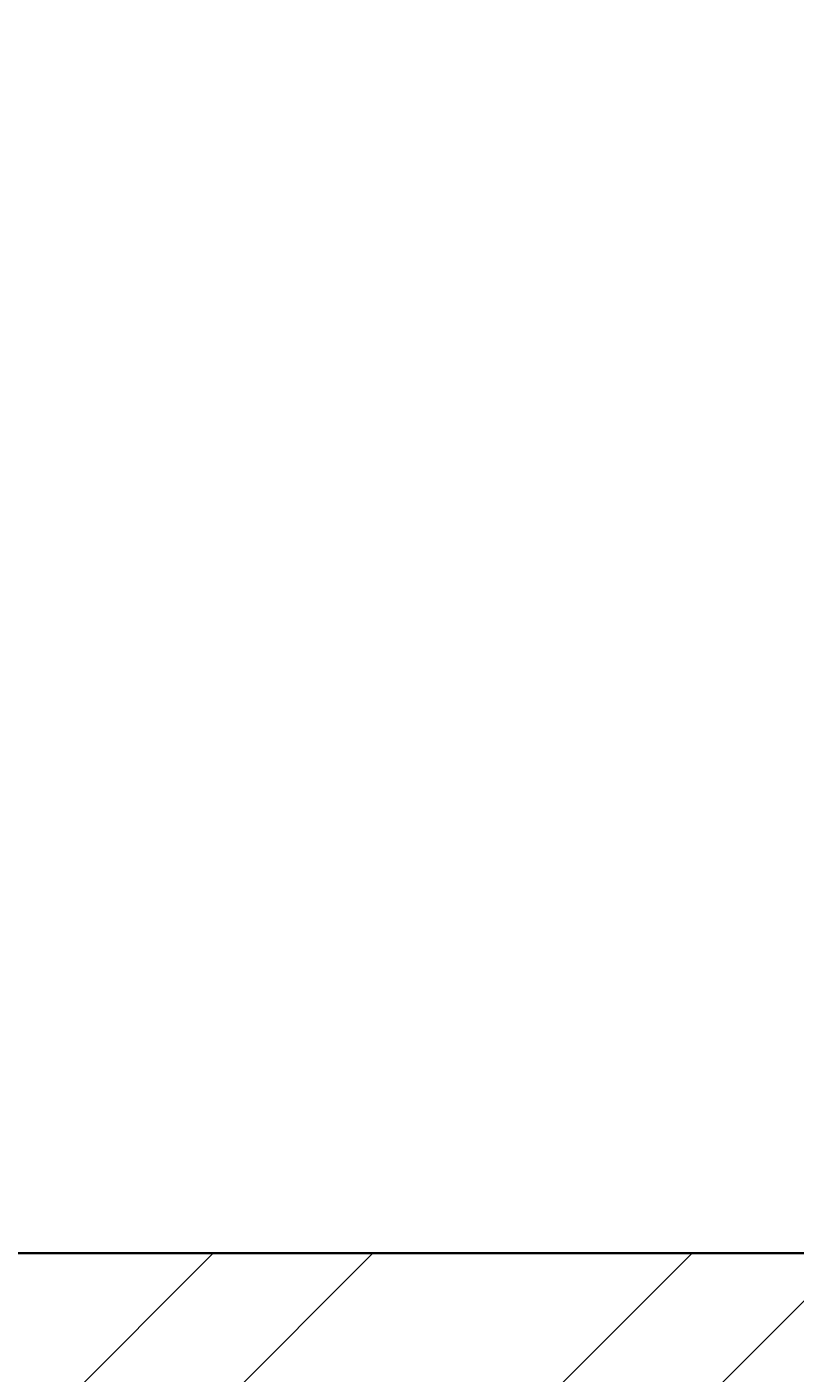
# Model space of a CAD drawing. Units: inches. Extents: x 1962 to 2771, y 1245 to 2660.
# Tile 52 of 114: x 2204 to 2225, y 2030 to 2068. Entities that reach past the tile are written whole.
import ezdxf

# ---------------------------------------------------------------- set-up
doc = ezdxf.new("R2010")
doc.units = ezdxf.units.IN
for name, color, linetype, lineweight in [('A-ANNO-DIMS', 2, 'Continuous', 18), ('A-WALL', 7, 'Continuous', 35), ('A-WALL-PATT', 252, 'Continuous', 13)]:
    doc.layers.add(name, color=color, linetype=linetype, lineweight=lineweight)
doc.styles.get("Standard").update_dxf_attribs({"font": 'arial.ttf'})
doc.dimstyles.get("Standard").update_dxf_attribs({"dimtxt": 0.18, "dimasz": 0.18, "dimexe": 0.18, "dimexo": 0.0625, "dimgap": 0.09, "dimtad": 0, "dimtih": 1, "dimtoh": 1, "dimdec": 4, "dimzin": 0, "dimdsep": 46, "dimtxsty": 'Standard', "dimcen": 0.09, "dimadec": 0, "dimazin": 0, "dimtfac": 1, "dimtdec": 4, "dimtofl": 0, "dimtmove": 0, "dimatfit": 3, "dimfxl": 1, "dimtolj": 1, "dimtzin": 0, "dimarcsym": 0})

# ---------------------------------------------------------------- blocks, each defined once
blk = doc.blocks.new('*D40')
at = {"layer": 'A-ANNO-DIMS', "color": 0, "lineweight": -2, "transparency": 16777216}
for p, q in [((2072.02, 2033.906), (2072.02, 2583.474)), ((2660.807, 2524.406), (2660.807, 2583.474)), ((2072.2, 2583.294), (2366.02, 2583.294)), ((2660.627, 2583.294), (2366.808, 2583.294))]:
    blk.add_line(p, q, dxfattribs=at)
at = {"layer": 'A-ANNO-DIMS', "color": 0, "transparency": 16777216}
for points in [[(2072.2, 2583.324), (2072.2, 2583.264), (2072.02, 2583.294)], [(2660.627, 2583.324), (2660.627, 2583.264), (2660.807, 2583.294)]]:
    blk.add_solid(points, dxfattribs=at)
at = {"layer": 'Defpoints', "color": 0, "transparency": 16777216}
for p in [(2660.807, 2583.294), (2660.807, 2524.344), (2072.02, 2033.844)]:
    blk.add_point(p, dxfattribs=at)
at = {"layer": 'A-ANNO-DIMS', "color": 0, "transparency": 16777216, "insert": (2366.414, 2583.294), "char_height": 0.18, "attachment_point": 5}
blk.add_mtext('\\A1;588.8', dxfattribs=at)

msp = doc.modelspace()

# ---------------------------------------------------------------- hatches: boundary and pattern name
at = {"layer": 'A-WALL-PATT'}
h = msp.add_hatch(dxfattribs=at)
h.set_pattern_fill('ANSI32', color=256)
h.paths.add_polyline_path([(2090.8074, 2467.3437), (2141.6481, 2467.3437), (2141.6481, 2469.5937), (2141.6481, 2471.8437), (2086.3074, 2471.8437), (2086.3074, 2422.5333), (2090.8074, 2422.5333)])
h.paths.add_polyline_path([(2282.7664, 2471.8437), (2204.8982, 2471.8437), (2204.8982, 2467.3437), (2234.8074, 2467.3437), (2234.8074, 2311.3437), (2228.7492, 2311.3437), (2228.7492, 2306.8437), (2234.8074, 2306.8437), (2331.9227, 2306.8437), (2331.9227, 2309.0937), (2331.9227, 2311.3437), (2239.3074, 2311.3437), (2239.3074, 2467.3437), (2282.7664, 2467.3437), (2282.7664, 2469.5937)])
h.paths.add_polyline_path([(2471.4531, 2519.8437), (2552.011, 2519.8437), (2564.3996, 2519.8437), (2564.3996, 2511.1389), (2568.8996, 2511.1389), (2568.8996, 2524.3437), (2466.9531, 2524.3437), (2466.9531, 2471.8437), (2450.0749, 2471.8437), (2446.4672, 2471.8437), (2446.4672, 2467.3437), (2450.0749, 2467.3437), (2475.9988, 2467.3437), (2475.9988, 2469.5937), (2475.9988, 2471.8437), (2471.4531, 2471.8437)])
h.paths.add_polyline_path([(2575.2231, 2469.5937), (2575.2231, 2471.8437), (2568.8996, 2471.8437), (2568.8996, 2487.1389), (2564.3996, 2487.1389), (2564.3996, 2471.8437), (2556.511, 2471.8437), (2499.2904, 2471.8437), (2499.2904, 2467.3437), (2507.8074, 2467.3437), (2507.8074, 2311.3437), (2414.863, 2311.3437), (2414.863, 2306.8437), (2512.3074, 2306.8437), (2517.0114, 2306.8437), (2517.0114, 2309.0937), (2517.0114, 2311.3437), (2512.3074, 2311.3437), (2512.3074, 2467.3437), (2575.2231, 2467.3437)])
h.paths.add_polyline_path([(2660.8074, 2471.8437), (2600.9602, 2471.8437), (2600.9602, 2467.3437), (2656.3074, 2467.3437), (2656.3074, 2432.5704), (2660.8074, 2432.5704)])
h.paths.add_polyline_path([(2660.8074, 2372.5704), (2656.3074, 2372.5704), (2656.3074, 2311.3437), (2600.276, 2311.3437), (2600.276, 2309.0937), (2600.276, 2306.8437), (2656.3074, 2306.8437), (2656.3074, 2296.2593), (2660.8074, 2296.2593)])
h.paths.add_polyline_path([(2572.3074, 2306.8437), (2577.1385, 2306.8437), (2577.1385, 2311.3437), (2551.082, 2311.3437), (2551.082, 2306.8437), (2567.8074, 2306.8437), (2567.8074, 2258.8437), (2540.0574, 2258.8437), (2540.0574, 2256.5937), (2540.0574, 2254.3437), (2567.8074, 2254.3437), (2656.3074, 2254.3437), (2656.3074, 2236.9085), (2660.8074, 2236.9085), (2660.8074, 2272.2593), (2656.3074, 2272.2593), (2656.3074, 2258.8437), (2572.3074, 2258.8437)])
h.paths.add_polyline_path([(2512.3074, 2254.3437), (2518.8716, 2254.3437), (2518.8716, 2256.5937), (2518.8716, 2258.8437), (2507.8074, 2258.8437), (2507.8074, 2177.8437), (2567.8074, 2177.8437), (2567.8074, 2172.9628), (2572.3074, 2172.9628), (2572.3074, 2177.8437), (2656.3074, 2177.8437), (2656.3074, 2166.4846), (2660.8074, 2166.4846), (2660.8074, 2200.9085), (2656.3074, 2200.9085), (2656.3074, 2182.3437), (2512.3074, 2182.3437)])
h.paths.add_polyline_path([(2656.3074, 2129.8437), (2572.3074, 2129.8437), (2572.3074, 2150.3044), (2570.0574, 2150.3044), (2567.8074, 2150.3044), (2567.8074, 2129.8437), (2507.8074, 2129.8437), (2507.8074, 2116.3027), (2510.0574, 2116.3027), (2512.3074, 2116.3027), (2512.3074, 2125.3437), (2567.8074, 2125.3437), (2572.3074, 2125.3437), (2656.3074, 2125.3437)])
h.paths.add_polyline_path([(2090.8074, 2362.5333), (2086.3074, 2362.5333), (2086.3074, 2298.6242), (2090.8074, 2298.6242), (2090.8074, 2306.8437), (2174.8074, 2306.8437), (2174.8074, 2286.4178), (2179.3074, 2286.4178), (2179.3074, 2306.8437), (2192.8641, 2306.8437), (2192.8641, 2309.0937), (2192.8641, 2311.3437), (2090.8074, 2311.3437)])
h.paths.add_polyline_path([(2209.156, 2258.8437), (2179.3074, 2258.8437), (2179.3074, 2263.2236), (2177.0574, 2263.2236), (2174.8074, 2263.2236), (2174.8074, 2258.8437), (2090.8074, 2258.8437), (2090.8074, 2274.6242), (2086.3074, 2274.6242), (2086.3074, 2238.2967), (2088.5574, 2238.2967), (2090.8074, 2238.2967), (2090.8074, 2254.3437), (2209.156, 2254.3437)])
h.paths.add_polyline_path([(2090.8074, 2177.8437), (2234.8074, 2177.8437), (2234.8074, 2173.1428), (2239.3074, 2173.1428), (2239.3074, 2258.8437), (2230.8442, 2258.8437), (2230.8442, 2256.5937), (2230.8442, 2254.3437), (2234.8074, 2254.3437), (2234.8074, 2182.3437), (2090.8074, 2182.3437), (2090.8074, 2202.2967), (2086.3074, 2202.2967), (2086.3074, 2140.0389), (2090.8074, 2140.0389)])
h.paths.add_polyline_path([(2090.8074, 2080.0389), (2086.3074, 2080.0389), (2086.3074, 2033.8437), (2090.8074, 2033.8437)], flags=17)
h.paths.add_polyline_path([(2244.9405, 2033.8437), (2239.3074, 2033.8437), (2239.3074, 2142.0665), (2237.2592, 2142.0665), (2234.8074, 2142.0665), (2234.8074, 2033.8437), (2090.8074, 2033.8437), (2076.5204, 2033.8437), (2072.0204, 2033.8437), (2072.0204, 2000.4493), (2076.5204, 2000.4493), (2076.5204, 2029.3437), (2090.8074, 2029.3437), (2244.9405, 2029.3437), (2244.9405, 2031.5937)])
h.paths.add_polyline_path([(2234.8074, 1933.3437), (2076.5204, 1933.3437), (2076.5204, 1952.4493), (2074.2704, 1952.4493), (2072.0204, 1952.4493), (2072.0204, 1933.3437), (2072.0204, 1928.8437), (2234.8074, 1928.8437)])
h.paths.add_polyline_path([(2090.8074, 1928.8437), (2086.3074, 1928.8437), (2086.3074, 1906.5013), (2090.8074, 1906.5013)])
h.paths.add_polyline_path([(2090.8074, 1846.5013), (2086.3074, 1846.5013), (2086.3074, 1769.9917), (2088.5574, 1769.9917), (2090.8074, 1769.9917), (2090.8074, 1780.3437), (2234.8074, 1780.3437), (2234.8074, 1708.3437), (2230.3764, 1708.3437), (2230.3764, 1703.8437), (2239.3074, 1703.8437), (2239.3074, 1792.6669), (2237.0574, 1792.6669), (2234.8074, 1792.6669), (2234.8074, 1784.8437), (2090.8074, 1784.8437)])
h.paths.add_polyline_path([(2239.3074, 1928.8437), (2244.9405, 1928.8437), (2244.9405, 1931.0937), (2244.9405, 1933.3437), (2234.8074, 1933.3437), (2234.8074, 1928.8437), (2234.8074, 1825.5949), (2239.3074, 1825.5949)])
h.paths.add_polyline_path([(2148.0425, 1649.0937), (2148.0425, 1651.3437), (2090.8074, 1651.3437), (2090.8074, 1646.8437), (2148.0425, 1646.8437)], flags=0)
h.paths.add_polyline_path([(2207.5601, 1708.3437), (2090.8074, 1708.3437), (2090.8074, 1703.8437), (2174.8074, 1703.8437), (2174.8074, 1651.3437), (2170.4457, 1651.3437), (2170.4457, 1646.8437), (2195.9924, 1646.8437), (2195.9924, 1649.0937), (2195.9924, 1651.3437), (2179.3074, 1651.3437), (2179.3074, 1703.8437), (2207.5601, 1703.8437), (2207.5601, 1706.0937)])
h.paths.add_polyline_path([(2090.8074, 1733.9917), (2086.3074, 1733.9917), (2086.3074, 1696.1032), (2088.5574, 1696.1032), (2090.8074, 1696.1032)])
h.paths.add_polyline_path([(2090.8074, 1672.1032), (2086.3074, 1672.1032), (2086.3074, 1600.3335), (2090.8074, 1600.3335)])
h.paths.add_polyline_path([(2090.8074, 1540.3335), (2086.3074, 1540.3335), (2086.3074, 1486.3437), (2139.6766, 1486.3437), (2139.6766, 1490.8437), (2090.8074, 1490.8437)])
h.paths.add_polyline_path([(2302.3876, 1490.8437), (2239.3074, 1490.8437), (2239.3074, 1646.8437), (2335.9994, 1646.8437), (2335.9994, 1651.3437), (2229.884, 1651.3437), (2229.884, 1646.8437), (2234.8074, 1646.8437), (2234.8074, 1490.8437), (2202.7103, 1490.8437), (2202.7103, 1488.5937), (2202.7103, 1486.3437), (2275.0699, 1486.3437), (2275.0699, 1475.772), (2279.5699, 1475.772), (2279.5699, 1486.3437), (2302.3876, 1486.3437)])
h.paths.add_polyline_path([(2279.5699, 1451.772), (2275.0699, 1451.772), (2275.0699, 1438.3437), (2174.8074, 1438.3437), (2174.8074, 1486.3437), (2179.7922, 1486.3437), (2179.7922, 1490.8437), (2163.3585, 1490.8437), (2163.3585, 1488.5937), (2163.3585, 1486.3437), (2170.3074, 1486.3437), (2170.3074, 1433.8437), (2279.5699, 1433.8437)])
h.paths.add_polyline_path([(2427.2363, 1490.8437), (2375.8074, 1490.8437), (2375.8074, 1646.8437), (2381.6401, 1646.8437), (2381.6401, 1651.3437), (2365.887, 1651.3437), (2365.887, 1649.0937), (2365.887, 1646.8437), (2371.3074, 1646.8437), (2371.3074, 1490.8437), (2327.5627, 1490.8437), (2327.5627, 1488.5937), (2327.5627, 1486.3437), (2371.3074, 1486.3437), (2371.3074, 1433.8437), (2375.8074, 1433.8437), (2375.8074, 1486.3437), (2427.2363, 1486.3437)])
h.paths.add_polyline_path([(2512.3074, 1646.8437), (2519.4351, 1646.8437), (2519.4351, 1649.0937), (2519.4351, 1651.3437), (2507.8074, 1651.3437), (2416.0063, 1651.3437), (2416.0063, 1649.0937), (2416.0063, 1646.8437), (2507.8074, 1646.8437), (2507.8074, 1490.8437), (2497.0532, 1490.8437), (2497.0532, 1488.5937), (2497.0532, 1486.3437), (2574.9344, 1486.3437), (2574.9344, 1476.0181), (2579.4344, 1476.0181), (2579.4344, 1486.3437), (2584.4872, 1486.3437), (2584.3074, 1490.8437), (2512.3074, 1490.8437)])
h.paths.add_polyline_path([(2470.5091, 1486.3437), (2473.9767, 1486.3437), (2473.9767, 1490.8437), (2449.6605, 1490.8437), (2449.6605, 1488.5937), (2449.6605, 1486.3437), (2466.0091, 1486.3437), (2466.0091, 1433.8437), (2470.5091, 1433.8437), (2579.4344, 1433.8437), (2579.4344, 1452.0181), (2574.9344, 1452.0181), (2574.9344, 1438.3437), (2554.5091, 1438.3437), (2470.5091, 1438.3437)])
h.paths.add_polyline_path([(2656.3074, 1490.8437), (2611.86, 1490.8437), (2611.86, 1486.3437), (2656.3074, 1486.3437)])
h.paths.add_polyline_path([(2660.8074, 1532.7007), (2658.5574, 1532.7007), (2656.3074, 1532.7007), (2656.3074, 1486.3437), (2660.8074, 1486.3437)])
h.paths.add_polyline_path([(2660.8074, 1664.9663), (2656.3074, 1664.9663), (2656.3074, 1651.3437), (2602.2313, 1651.3437), (2602.2313, 1646.8437), (2656.3074, 1646.8437), (2656.3074, 1592.7007), (2660.8074, 1592.7007)])
h.paths.add_polyline_path([(2660.8074, 1724.5221), (2656.3074, 1724.5221), (2656.3074, 1703.8437), (2542.4725, 1703.8437), (2542.4725, 1699.3437), (2567.8074, 1699.3437), (2567.8074, 1651.3437), (2552.7766, 1651.3437), (2552.7766, 1649.0937), (2552.7766, 1646.8437), (2577.2878, 1646.8437), (2577.2878, 1649.0937), (2577.2878, 1651.3437), (2572.3074, 1651.3437), (2572.3074, 1699.3437), (2656.3074, 1699.3437), (2656.3074, 1688.9663), (2660.8074, 1688.9663)])
h.paths.add_polyline_path([(2660.8074, 1880.6524), (2656.3074, 1880.6524), (2656.3074, 1832.8437), (2512.3074, 1832.8437), (2512.3074, 1837.8959), (2507.8074, 1837.8959), (2507.8074, 1828.3437), (2567.8074, 1828.3437), (2567.8074, 1804.3437), (2572.3074, 1804.3437), (2572.3074, 1828.3437), (2656.3074, 1828.3437), (2656.3074, 1818.6778), (2660.8074, 1818.6778)])
h.paths.add_polyline_path([(2660.8074, 1794.6778), (2656.3074, 1794.6778), (2656.3074, 1780.3437), (2572.3074, 1780.3437), (2572.3074, 1783.0303), (2570.0574, 1783.0303), (2567.8074, 1783.0303), (2567.8074, 1780.3437), (2507.8074, 1780.3437), (2507.8074, 1699.3437), (2517.8858, 1699.3437), (2517.8858, 1701.5937), (2517.8858, 1703.8437), (2512.3074, 1703.8437), (2512.3074, 1775.8437), (2656.3074, 1775.8437), (2656.3074, 1760.5221), (2660.8074, 1760.5221)])
h.paths.add_polyline_path([(2660.8074, 1981.3437), (2660.8074, 2020.2808), (2658.5574, 2020.2808), (2656.3074, 2020.2808), (2656.3074, 1981.3437), (2512.3074, 1981.3437), (2512.3074, 2086.6996), (2507.8074, 2086.6996), (2507.8074, 1981.3437), (2375.8074, 1981.3437), (2375.8074, 1986.8505), (2373.5574, 1986.8505), (2371.3074, 1986.8505), (2371.3074, 1973.2607), (2375.8074, 1973.2607), (2375.8074, 1976.8437), (2507.8074, 1976.8437), (2507.8074, 1865.4281), (2510.0574, 1865.4281), (2512.3074, 1865.4281), (2512.3074, 1976.8437), (2660.8074, 1976.8437)])
h.paths.add_polyline_path([(2375.8074, 1940.297), (2373.5574, 1940.297), (2371.3074, 1940.297), (2371.3074, 1933.3437), (2278.4434, 1933.3437), (2278.4434, 1928.8437), (2371.3074, 1928.8437), (2371.3074, 1651.3437), (2375.8074, 1651.3437)])
h.paths.add_polyline_path([(2660.8074, 1976.8437), (2656.3074, 1976.8437), (2656.3074, 1940.6524), (2660.8074, 1940.6524)], flags=17)
h.paths.add_polyline_path([(2660.8074, 2142.4846), (2656.3074, 2142.4846), (2656.3074, 2080.2808), (2660.8074, 2080.2808)])
h.paths.add_polyline_path([(2381.4189, 2311.3437), (2375.8074, 2311.3437), (2375.8074, 2467.3437), (2424.7242, 2467.3437), (2424.7242, 2469.5937), (2424.7242, 2471.8437), (2375.8074, 2471.8437), (2375.8074, 2524.3437), (2371.3074, 2524.3437), (2371.3074, 2471.8437), (2307.2097, 2471.8437), (2307.2097, 2467.3437), (2371.3074, 2467.3437), (2371.3074, 2311.3437), (2366.8901, 2311.3437), (2366.8901, 2306.8437), (2371.3074, 2306.8437), (2371.3074, 2033.8437), (2279.6589, 2033.8437), (2279.6589, 2029.3437), (2371.3074, 2029.3437), (2371.3074, 2014.2598), (2375.8074, 2014.2598), (2375.8074, 2306.8437), (2381.4189, 2306.8437)])
h.paths.add_polyline_path([(2263.3074, 2524.3437), (2170.3074, 2524.3437), (2170.3074, 2519.8437), (2170.3074, 2471.8437), (2165.0312, 2471.8437), (2165.0312, 2467.3437), (2179.6721, 2467.3437), (2179.6721, 2469.5161), (2179.6721, 2471.8437), (2174.8074, 2471.8437), (2174.8074, 2519.8437), (2258.8074, 2519.8437), (2258.8074, 2511.6436), (2263.3074, 2511.6436)])
h.paths.add_polyline_path([(2245.0232, 1361.4123), (2492.9468, 1361.4123), (2492.9468, 1398.505), (2245.0232, 1398.505)], flags=9)
h.paths.add_polyline_path([(2388.1434, 2086.6936), (2425.0704, 2086.6936), (2425.0704, 2105.3509), (2388.1434, 2105.3509)], flags=9)
h.paths.add_polyline_path([(2404.922, 2242.6744), (2445.7337, 2242.6744), (2445.7337, 2261.3318), (2404.922, 2261.3318)], flags=9)
h.paths.add_polyline_path([(2269.4107, 2156.7935), (2306.3378, 2156.7935), (2306.3378, 2175.4508), (2269.4107, 2175.4508)], flags=9)
h.paths.add_polyline_path([(2269.3277, 2233.4343), (2306.2547, 2233.4343), (2306.2547, 2252.0917), (2269.3277, 2252.0917)], flags=9)
h.paths.add_polyline_path([(2431.6052, 2320.6922), (2470.4456, 2320.6922), (2470.4456, 2339.3495), (2431.6052, 2339.3495)], flags=25)
h.paths.add_polyline_path([(2249.6902, 2315.7608), (2288.5306, 2315.7608), (2288.5306, 2334.4182), (2249.6902, 2334.4182)], flags=25)
h.paths.add_polyline_path([(2096.9301, 2314.3181), (2135.7704, 2314.3181), (2135.7704, 2332.9755), (2096.9301, 2332.9755)], flags=25)
h.paths.add_polyline_path([(2134.3475, 2285.7089), (2161.4655, 2285.7089), (2161.4655, 2304.3662), (2134.3475, 2304.3662)], flags=9)
h.paths.add_polyline_path([(2126.5155, 2209.4076), (2159.9227, 2209.4076), (2159.9227, 2228.065), (2126.5155, 2228.065)], flags=25)
h.paths.add_polyline_path([(2110.5753, 2141.5299), (2149.4157, 2141.5299), (2149.4157, 2160.1872), (2110.5753, 2160.1872)], flags=25)
h.paths.add_polyline_path([(2249.8618, 1968.3317), (2286.3966, 1968.3317), (2286.3966, 1986.989), (2249.8618, 1986.989)], flags=9)
h.paths.add_polyline_path([(2395.9507, 1777.0051), (2436.7624, 1777.0051), (2436.7624, 1795.6625), (2395.9507, 1795.6625)], flags=9)
h.paths.add_polyline_path([(2398.5259, 1888.5651), (2435.0062, 1888.5651), (2435.0062, 1907.2224), (2398.5259, 1907.2224)], flags=25)
h.paths.add_polyline_path([(2259.3506, 1728.3559), (2296.2776, 1728.3559), (2296.2776, 1747.0132), (2259.3506, 1747.0132)], flags=9)
h.paths.add_polyline_path([(2271.3698, 1845.268), (2308.2968, 1845.268), (2308.2968, 1863.9253), (2271.3698, 1863.9253)], flags=9)
h.paths.add_polyline_path([(2120.9355, 1786.3027), (2159.7759, 1786.3027), (2159.7759, 1804.9601), (2120.9355, 1804.9601)], flags=25)
h.paths.add_polyline_path([(2121.3164, 1732.1043), (2154.7236, 1732.1043), (2154.7236, 1750.7616), (2121.3164, 1750.7616)], flags=25)
h.paths.add_polyline_path([(2118.3706, 1678.8997), (2147.5282, 1678.8997), (2147.5282, 1697.557), (2118.3706, 1697.557)], flags=25)
h.paths.add_polyline_path([(2385.9227, 1493.557), (2424.763, 1493.557), (2424.763, 1512.2143), (2385.9227, 1512.2143)], flags=25)
h.paths.add_polyline_path([(2248.7058, 1500.0256), (2287.5462, 1500.0256), (2287.5462, 1518.6829), (2248.7058, 1518.6829)], flags=25)
h.paths.add_polyline_path([(2104.1669, 1617.3771), (2143.0073, 1617.3771), (2143.0073, 1636.0344), (2104.1669, 1636.0344)], flags=9)
h.paths.add_polyline_path([(2096.0714, 1447.8824), (2137.3845, 1447.8824), (2137.3845, 1458.1859), (2096.0714, 1458.1859)], flags=9)
h.paths.add_polyline_path([(2180.6114, 1440.325), (2209.7689, 1440.325), (2209.7689, 1458.9823), (2180.6114, 1458.9823)], flags=25)
h.paths.add_polyline_path([(2316.1698, 1447.9637), (2357.4829, 1447.9637), (2357.4829, 1458.2673), (2316.1698, 1458.2673)], flags=9)
h.paths.add_polyline_path([(2397.6187, 1447.9637), (2438.9318, 1447.9637), (2438.9318, 1458.2673), (2397.6187, 1458.2673)], flags=9)
h.paths.add_polyline_path([(2473.0778, 1439.5953), (2502.2354, 1439.5953), (2502.2354, 1458.2527), (2473.0778, 1458.2527)], flags=25)
h.paths.add_polyline_path([(2589.7027, 1447.8819), (2631.0158, 1447.8819), (2631.0158, 1458.1855), (2589.7027, 1458.1855)], flags=9)
h.paths.add_polyline_path([(2522.4009, 1497.5285), (2561.2413, 1497.5285), (2561.2413, 1516.1859), (2522.4009, 1516.1859)], flags=25)
h.paths.add_polyline_path([(2579.6565, 1671.3482), (2608.8141, 1671.3482), (2608.8141, 1690.0056), (2579.6565, 1690.0056)], flags=25)
h.paths.add_polyline_path([(2544.7038, 1725.5064), (2578.1111, 1725.5064), (2578.1111, 1744.1637), (2544.7038, 1744.1637)], flags=25)
h.paths.add_polyline_path([(2578.1191, 1807.472), (2607.2766, 1807.472), (2607.2766, 1826.1293), (2578.1191, 1826.1293)], flags=25)
h.paths.add_polyline_path([(2595.0614, 1835.1839), (2633.9018, 1835.1839), (2633.9018, 1853.8413), (2595.0614, 1853.8413)], flags=25)
h.paths.add_polyline_path([(2567.0097, 2097.7035), (2605.8501, 2097.7035), (2605.8501, 2116.3609), (2567.0097, 2116.3609)], flags=9)
h.paths.add_polyline_path([(2586.644, 2134.6454), (2615.8015, 2134.6454), (2615.8015, 2153.3027), (2586.644, 2153.3027)], flags=9)
h.paths.add_polyline_path([(2544.6185, 2212.6783), (2578.0258, 2212.6783), (2578.0258, 2231.3356), (2544.6185, 2231.3356)], flags=25)
h.paths.add_polyline_path([(2577.0273, 2256.9023), (2606.1849, 2256.9023), (2606.1849, 2275.5597), (2577.0273, 2275.5597)], flags=24)
h.paths.add_polyline_path([(2605.2683, 2315.2821), (2644.1087, 2315.2821), (2644.1087, 2333.9395), (2605.2683, 2333.9395)], flags=25)
h.paths.add_polyline_path([(2583.1244, 2496.1815), (2624.4375, 2496.1815), (2624.4375, 2506.4851), (2583.1244, 2506.4851)], flags=9)
h.paths.add_polyline_path([(2474.761, 2497.0823), (2503.9185, 2497.0823), (2503.9185, 2515.7397), (2474.761, 2515.7397)], flags=25)
h.paths.add_polyline_path([(2387.5787, 2494.2563), (2428.902, 2494.2563), (2428.902, 2504.5598), (2387.5787, 2504.5598)], flags=9)
h.paths.add_polyline_path([(2300.1657, 2500.1564), (2341.4788, 2500.1564), (2341.4788, 2510.46), (2300.1657, 2510.46)], flags=25)
h.paths.add_polyline_path([(2176.8589, 2497.5843), (2206.0165, 2497.5843), (2206.0165, 2516.2416), (2176.8589, 2516.2416)], flags=25)
h.paths.add_polyline_path([(2097.4668, 2494.9762), (2138.7799, 2494.9762), (2138.7799, 2505.2798), (2097.4668, 2505.2798)], flags=9)

# ---------------------------------------------------------------- linework, layer by layer
at = {"layer": 'A-WALL'}
msp.add_line((2090.8074, 2033.8437), (2234.8074, 2033.8437), dxfattribs=at)

# ---------------------------------------------------------------- dimensions: what is measured, and where the dimension line sits
at = {"layer": 'A-ANNO-DIMS'}
dim = msp.add_linear_dim(base=(2660.8074, 2583.2937), p1=(2072.0204, 2033.8437), p2=(2660.8074, 2524.3437), dimstyle='Standard', override={"dimdec": 1, "dimlfac": 1, "dimrnd": 0, "dimzin": 0, "dimdsep": 46, "dimlunit": 2}, dxfattribs=at)
dim.commit()
dim.dimension.update_dxf_attribs({"geometry": '*D40', "text_midpoint": (2366.4139, 2583.2937)})

doc.saveas('drawing.dxf')
